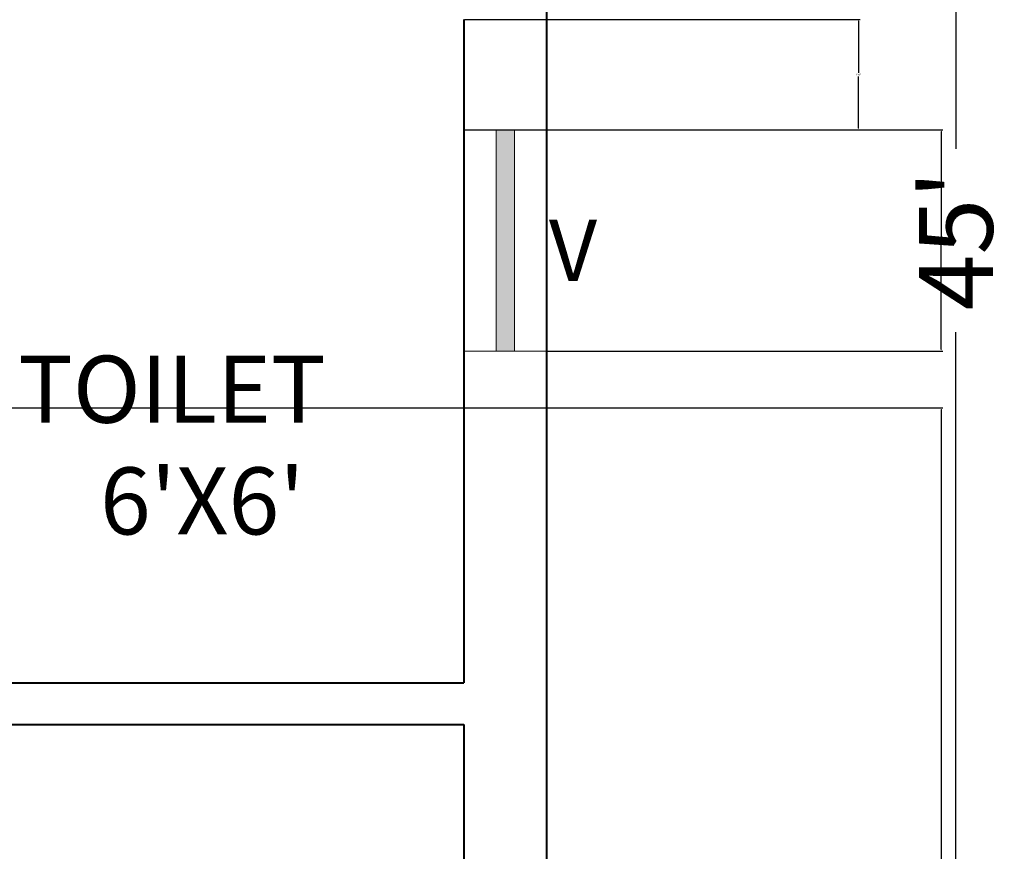
# Model space of a CAD drawing. Units: inches. Extents: x 182 to 1022, y -617 to 111.
# Tile 30 of 33: x 915 to 1022, y -337 to -246. Entities that reach past the tile are written whole.
import ezdxf

# ---------------------------------------------------------------- set-up
doc = ezdxf.new("R2010")
doc.units = ezdxf.units.IN
doc.header["$MEASUREMENT"] = 0
for name, color, linetype, lineweight in [('A-ANNO-DIMS', 2, 'Continuous', 18), ('A-ANNO-IDEN', 1, 'Continuous', 18), ('A-AREA-IDEN', 8, 'Continuous', 18), ('A-GLAZ-PATT', 5, 'Continuous', 13), ('wall', 1, 'Continuous', 40), ('wind', 5, 'Continuous', 20)]:
    doc.layers.add(name, color=color, linetype=linetype, lineweight=lineweight)
doc.styles.get("Standard").update_dxf_attribs({"font": 'arial.ttf'})
doc.dimstyles.get("Standard").update_dxf_attribs({"dimtxt": 0.18, "dimasz": 0.18, "dimexe": 0.18, "dimexo": 0.0625, "dimgap": 0.09, "dimtad": 0, "dimtih": 1, "dimtoh": 1, "dimdec": 1, "dimzin": 0, "dimdsep": 46, "dimlunit": 4, "dimtxsty": 'Standard', "dimcen": 0.09, "dimadec": 0, "dimazin": 0, "dimtfac": 1, "dimtdec": 1, "dimtofl": 0, "dimtmove": 0, "dimatfit": 3, "dimfxl": 1, "dimtolj": 1, "dimtzin": 0, "dimarcsym": 0})

# ---------------------------------------------------------------- blocks, each defined once
blk = doc.blocks.new('_ArchTick')
at = {"color": 0, "linetype": 'ByBlock', "const_width": 0.15}
blk.add_lwpolyline([(-0.5, -0.5), (0.5, 0.5)], dxfattribs=at)
blk = doc.blocks.new('*D8')
at = {"layer": 'A-ANNO-DIMS', "color": 0, "lineweight": -2, "transparency": 16777216}
for p, q in [((1016.69, -0.37), (1016.69, -260.42)), ((1016.69, -540.37), (1016.69, -280.32))]:
    blk.add_line(p, q, dxfattribs=at)
at = {"layer": 'Defpoints', "color": 0, "transparency": 16777216}
for p in [(972.3, -0.37), (972.3, -540.37), (1016.69, -540.37)]:
    blk.add_point(p, dxfattribs=at)
at = {"layer": 'A-ANNO-DIMS', "color": 0, "lineweight": -2, "transparency": 16777216, "xscale": 8, "yscale": 8, "zscale": 8}
for p, rotation in [((1016.69, -0.37), 90), ((1016.69, -540.37), 270)]:
    blk.add_blockref('_ArchTick', p, dxfattribs=dict(at, rotation=rotation))
at = {"layer": 'A-ANNO-DIMS', "color": 0, "transparency": 16777216, "insert": (1016.69, -270.37), "char_height": 8, "attachment_point": 5, "rotation": 90}
blk.add_mtext("\\A1;45'", dxfattribs=at)
blk = doc.blocks.new('*D37')
at = {"layer": 'A-ANNO-DIMS', "color": 0, "lineweight": -2, "transparency": 16777216}
for p, q in [((963.37, -246.37), (1006.28, -246.37)), ((1006.1, -246.55), (1006.1, -252.19)), ((1006.1, -258.19), (1006.1, -252.56)), ((963.37, -258.37), (1006.28, -258.37))]:
    blk.add_line(p, q, dxfattribs=at)
at = {"layer": 'A-ANNO-DIMS', "color": 0, "transparency": 16777216}
for points in [[(1006.07, -246.55), (1006.13, -246.55), (1006.1, -246.37)], [(1006.07, -258.19), (1006.13, -258.19), (1006.1, -258.37)]]:
    blk.add_solid(points, dxfattribs=at)
at = {"layer": 'Defpoints', "color": 0, "transparency": 16777216}
for p in [(963.3, -246.37), (963.3, -258.37), (1006.1, -258.37)]:
    blk.add_point(p, dxfattribs=at)
at = {"layer": 'A-ANNO-DIMS', "color": 0, "transparency": 16777216, "insert": (1006.1, -252.37), "char_height": 0.18, "attachment_point": 5}
blk.add_mtext('\\A1;1\'-0"', dxfattribs=at)
blk = doc.blocks.new('*D38')
at = {"layer": 'A-ANNO-DIMS', "color": 0, "lineweight": -2, "transparency": 16777216}
for p, q in [((972.37, -258.37), (1015.28, -258.37)), ((1015.1, -258.55), (1015.1, -270.19)), ((1015.1, -282.19), (1015.1, -270.56)), ((972.37, -282.37), (1015.28, -282.37))]:
    blk.add_line(p, q, dxfattribs=at)
at = {"layer": 'A-ANNO-DIMS', "color": 0, "transparency": 16777216}
for points in [[(1015.07, -258.55), (1015.13, -258.55), (1015.1, -258.37)], [(1015.07, -282.19), (1015.13, -282.19), (1015.1, -282.37)]]:
    blk.add_solid(points, dxfattribs=at)
at = {"layer": 'Defpoints', "color": 0, "transparency": 16777216}
for p in [(972.3, -258.37), (972.3, -282.37), (1015.1, -282.37)]:
    blk.add_point(p, dxfattribs=at)
at = {"layer": 'A-ANNO-DIMS', "color": 0, "transparency": 16777216, "insert": (1015.1, -270.37), "char_height": 0.18, "attachment_point": 5}
blk.add_mtext('\\A1;2\'-0"', dxfattribs=at)
blk = doc.blocks.new('*D39')
at = {"layer": 'A-ANNO-DIMS', "color": 0, "lineweight": -2, "transparency": 16777216}
for p, q in [((238.4, -288.54), (1015.28, -288.54)), ((1015.1, -288.72), (1015.1, -346.77)), ((1015.1, -405.19), (1015.1, -347.14)), ((238.43, -405.37), (1015.28, -405.37))]:
    blk.add_line(p, q, dxfattribs=at)
at = {"layer": 'A-ANNO-DIMS', "color": 0, "transparency": 16777216}
for points in [[(1015.07, -288.72), (1015.13, -288.72), (1015.1, -288.54)], [(1015.07, -405.19), (1015.13, -405.19), (1015.1, -405.37)]]:
    blk.add_solid(points, dxfattribs=at)
at = {"layer": 'Defpoints', "color": 0, "transparency": 16777216}
for p in [(238.34, -288.54), (1015.1, -288.54), (238.36, -405.37)]:
    blk.add_point(p, dxfattribs=at)
at = {"layer": 'A-ANNO-DIMS', "color": 0, "transparency": 16777216, "insert": (1015.1, -346.96), "char_height": 0.18, "attachment_point": 5}
blk.add_mtext('\\A1;9\'-9"', dxfattribs=at)

msp = doc.modelspace()

# ---------------------------------------------------------------- hatches: boundary and pattern name
at = {"layer": 'A-GLAZ-PATT'}
h = msp.add_hatch(color=256, dxfattribs=at)
h.dxf.hatch_style = 1
h.paths.add_polyline_path([(692.35, -3.87), (662.35, -3.87), (662.35, -5.87), (692.35, -5.87)])
h.paths.add_polyline_path([(783.03, -3.87), (747.03, -3.87), (747.03, -5.87), (783.03, -5.87)])
h.paths.add_polyline_path([(641.8, -252.37), (639.8, -252.37), (639.8, -288.37), (641.8, -288.37)])
h.paths.add_polyline_path([(968.8, -258.37), (966.8, -258.37), (966.8, -282.37), (968.8, -282.37)])
h.paths.add_polyline_path([(968.8, -132.92), (966.8, -132.92), (966.8, -168.92), (968.8, -168.92)])
h.paths.add_polyline_path([(940.3, -534.87), (904.3, -534.87), (904.3, -536.87), (940.3, -536.87)])

# ---------------------------------------------------------------- linework, layer by layer
at = {"layer": 'wall'}
for p, q in [((972.3, -540.37), (972.3, -0.37)), ((963.3, -246.37), (963.3, -318.37)), ((891.3, -318.37), (963.3, -318.37)), ((886.8, -322.87), (963.3, -322.87)), ((963.3, -322.87), (963.3, -531.37))]:
    msp.add_line(p, q, dxfattribs=at)
at = {"layer": 'wind'}
for p, q in [((963.3, -258.37), (972.3, -258.37)), ((966.8, -258.37), (966.8, -282.37)), ((968.8, -258.37), (968.8, -282.37)), ((963.3, -282.37), (972.3, -282.37))]:
    msp.add_line(p, q, dxfattribs=at)

# ---------------------------------------------------------------- texts
at = {"layer": 'A-ANNO-IDEN'}
msp.add_text('V', height=6.65, dxfattribs=at).set_placement((972.53, -274.77))
at = {"layer": 'A-AREA-IDEN', "insert": (914.94, -282.87), "char_height": 7.2703, "attachment_point": 1}
msp.add_mtext_dynamic_manual_height_columns("TOILET        6'X6'", width=40.102, gutter_width=1.21, heights=[0], dxfattribs=at)

# ---------------------------------------------------------------- dimensions: what is measured, and where the dimension line sits
at = {"layer": 'A-ANNO-DIMS'}
for base, p1, p2, angle, override, picture, middle in [((1016.69, -540.37), (972.3, -0.37), (972.3, -540.37), 90, {"dimtxt": 8, "dimasz": 8, "dimgap": 3, "dimtih": 0, "dimblk1": 'ArchTick', "dimblk2": 'ArchTick', "dimsah": 1, "dimse1": 1, "dimse2": 1, "dimclrd": 0, "dimclre": 0, "dimclrt": 0}, '*D8', (1016.69, -270.37)), ((1006.1, -258.37), (963.3, -246.37), (963.3, -258.37), 270, {"dimdec": 1, "dimlfac": 1, "dimrnd": 0, "dimzin": 1, "dimdsep": 46, "dimlunit": 4, "dimfrac": 2}, '*D37', (1006.1, -252.37)), ((1015.1, -282.37), (972.3, -258.37), (972.3, -282.37), 270, {"dimdec": 1, "dimlfac": 1, "dimrnd": 0, "dimzin": 1, "dimdsep": 46, "dimlunit": 4, "dimfrac": 2}, '*D38', (1015.1, -270.37)), ((1015.1, -288.54), (238.36, -405.37), (238.34, -288.54), 90, {"dimdec": 1, "dimlfac": 1, "dimrnd": 0, "dimzin": 1, "dimdsep": 46, "dimlunit": 4, "dimfrac": 2}, '*D39', (1015.1, -346.96))]:
    dim = msp.add_linear_dim(base=base, p1=p1, p2=p2, angle=angle, dimstyle='Standard', override=override, dxfattribs=at)
    dim.commit()
    dim.dimension.update_dxf_attribs({"geometry": picture, "text_midpoint": middle})

doc.saveas('drawing.dxf')
